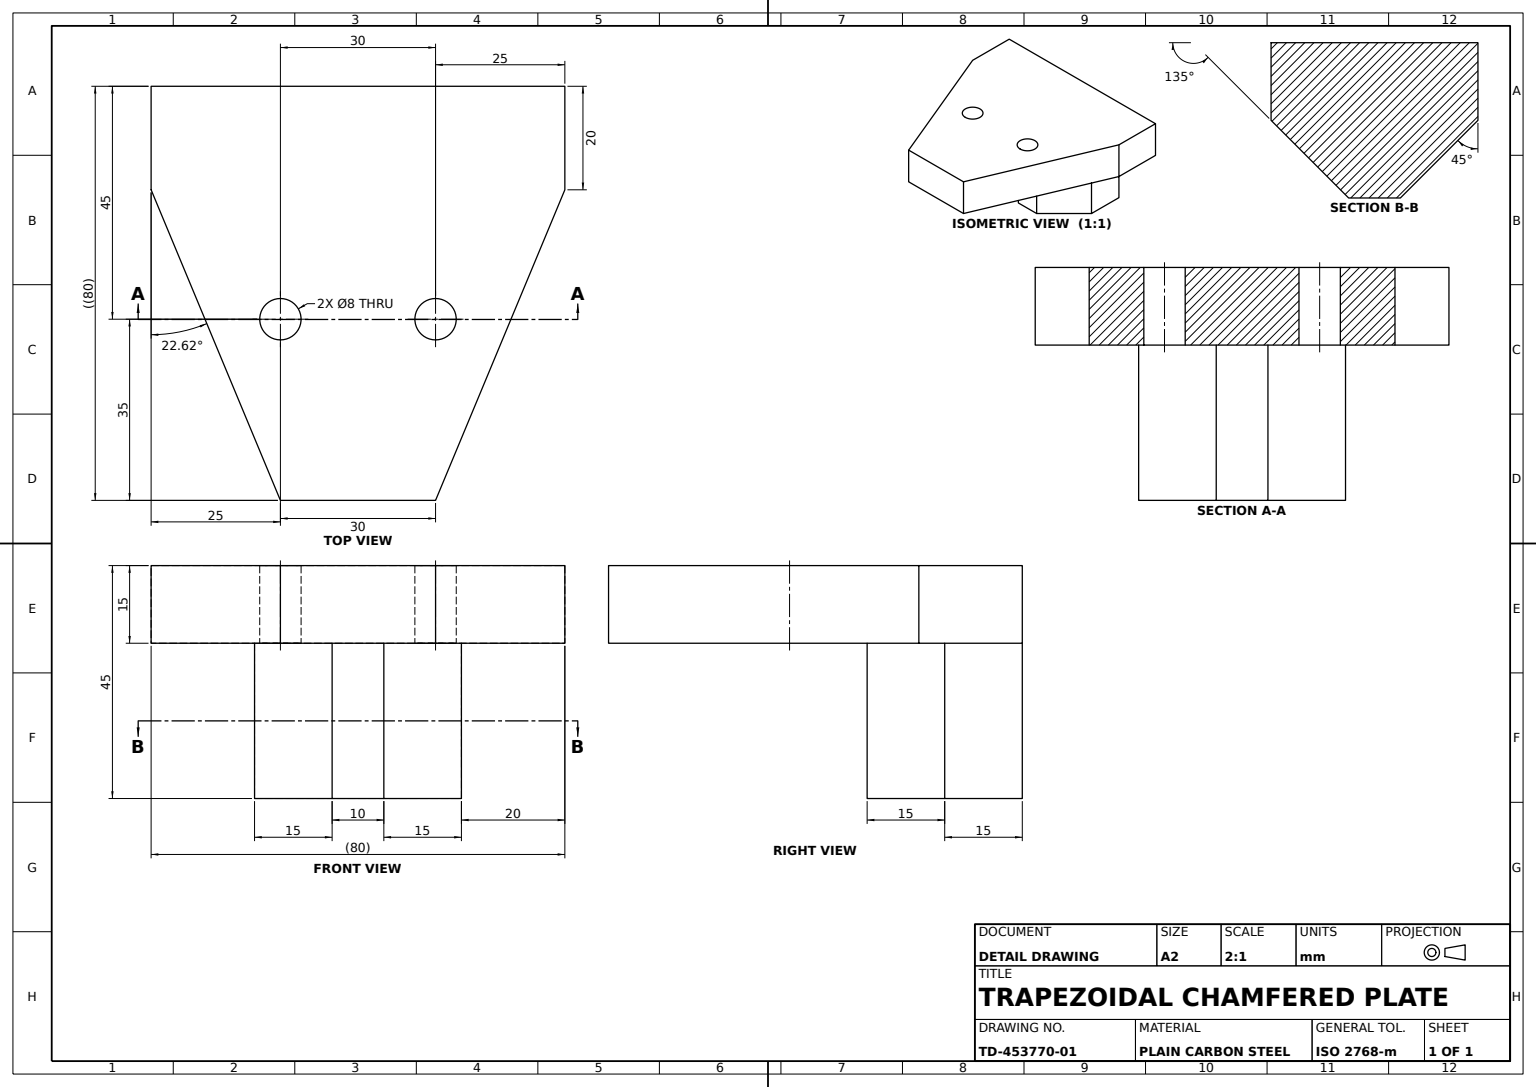
SolidWorks part; units mm, degrees
material "Plain Carbon Steel"
ref_plane "Front Plane" through (0, 0, 0) normal (0, 0, 1) x (1, 0, 0)
ref_plane "Top Plane" through (0, 0, 0) normal (0, 1, 0) x (1, 0, 0)
ref_plane "Right Plane" through (0, 0, 0) normal (1, 0, 0) x (0, 0, -1)
sketch "Base Plate Sketch" plane through (0, 0, 0) normal (0, 0, 1) x (1, 0, 0)
  line L0 (0, 0) -> (80, 0)
  line L1 (80, 0) -> (80, 10)
  line L2 (80, 10) -> (0, 10)
  line L3 (0, 10) -> (0, 0)
  dimension "D1" = 80
  dimension "D2" = 10
extrude "Base Plate" add sketch "Base Plate Sketch" along normal blind 20
sketch "Pentagonal Boss Sketch" plane through (0, 0, 0) normal (0, -1, 0) x (1, 0, 0)
  line L0 (80, 20) -> (80, 0) construction
  line L1 (0, 0) -> (80, 0) construction
  line L2 (40, 80) -> (25, 80)
  line L3 (40, 80) -> (55, 80)
  line L4 (55, 80) -> (80, 20)
  line L5 (80, 20) -> (0, 20)
  line L6 (0, 20) -> (25, 80)
  dimension "D1" = 25
  dimension "D2" = 80
extrude "Pentagonal Boss" add sketch "Pentagonal Boss Sketch" against normal blind 15
sketch "Four-Sided Boss Sketch" plane through (0, 0, 0) normal (0, 0, -1) x (-1, 0, 0)
  line L0 (-80, 10) -> (-80, 15)
  line L1 (-80, 15) -> (0, 15)
  line L2 (0, 15) -> (0, 10)
  line L3 (0, 10) -> (-80, 10)
extrude "Four-Sided Boss" add sketch "Four-Sided Boss Sketch" against normal blind 20
sketch "Octagonal Boss Sketch" plane through (0, 0, 0) normal (0, -1, 0) x (1, 0, 0)
  line L0 (40, 0) -> (60, 0)
  line L1 (0, 0) -> (80, 0) construction
  line L2 (60, 0) -> (60, 15)
  line L3 (40, 0) -> (20, 0)
  line L4 (20, 0) -> (20, 15)
  line L6 (40, 30) -> (35, 30)
  line L7 (35, 30) -> (20, 15)
  line L8 (40, 30) -> (45, 30)
  line L9 (45, 30) -> (60, 15)
  line L10 (80, 20) -> (80, 0) construction
  dimension "D1" = 20
  dimension "D2" = 35
  dimension "D3" = 15
extrude "Octagonal Boss" add sketch "Octagonal Boss Sketch" along normal blind 30
sketch "Holes 2xØ8 Sketch" plane through (0, 0, 0) normal (0, -1, 0) x (1, 0, 0)
  line L0 (20, 15) -> (20, 0) construction
  circle A0 centre (25, 45) radius 4
  circle A1 centre (55, 45) radius 4
  dimension "D1" = 8
  dimension "D2" = 8
  dimension "D3" = 8
  dimension "D4" = 5
  dimension "D5" = 35
  dimension "D6" = 45
extrude "Holes 2xØ8" cut sketch "Holes 2xØ8 Sketch" against normal blind 15
